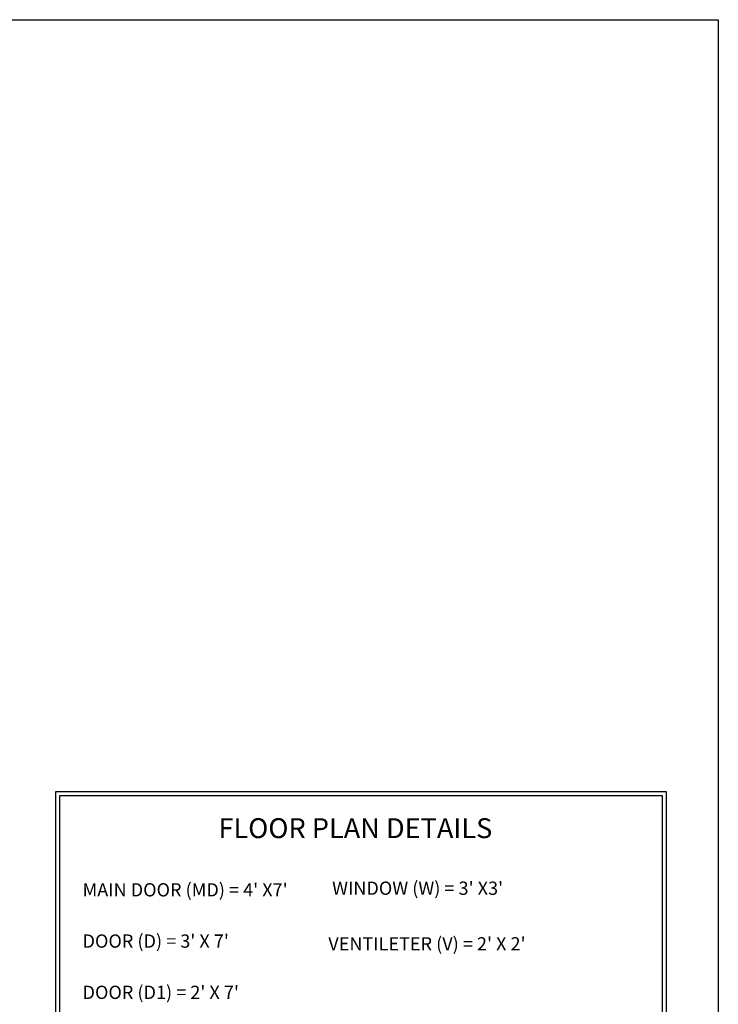
# Model space of a CAD drawing. Units: inches. Extents: x 1662 to 23131, y 1265 to 19127.
# Tile 26 of 26: x 22604 to 23131, y 18361 to 19104. Entities that reach past the tile are written whole.
import ezdxf

# ---------------------------------------------------------------- set-up
doc = ezdxf.new("R2010")
doc.units = ezdxf.units.IN
for name, color, linetype, lineweight in [('A-ANNO-TEXT', 7, 'Continuous', 18), ('A-ANNO-TITL', 7, 'Continuous', 35), ('A-ANNO-TTLB', 7, 'Continuous', 25)]:
    doc.layers.add(name, color=color, linetype=linetype, lineweight=lineweight)
doc.styles.get("Standard").update_dxf_attribs({"font": 'arial.ttf'})

# ---------------------------------------------------------------- blocks, each defined once
blk = doc.blocks.new('SCHEDULE-FRAME')
for points in [[(0, 206.36), (460.01, 206.36), (460.01, 0), (0, 0)], [(3, 203.36), (457.01, 203.36), (457.01, 3), (3, 3)]]:
    blk.add_lwpolyline(points, close=True)

msp = doc.modelspace()

# ---------------------------------------------------------------- linework, layer by layer
at = {"layer": 'A-ANNO-TTLB'}
msp.add_lwpolyline([(21860.989, 19103.605), (23130.86, 19103.605), (23130.86, 17867.351), (21860.989, 17867.351)], close=True, dxfattribs=at)

# ---------------------------------------------------------------- block references
msp.add_blockref('SCHEDULE-FRAME', (22631.532, 18315.105), dxfattribs=at)

# ---------------------------------------------------------------- texts
at = {"layer": 'A-ANNO-TEXT', "char_height": 10, "attachment_point": 1}
for s, insert in [("MAIN DOOR (MD) = 4' X7'", (22651.685, 18452.431)), ("WINDOW (W) = 3' X3'", (22839.8, 18453.651)), ("DOOR (D) = 3' X 7'", (22651.685, 18413.779)), ("VENTILETER (V) = 2' X 2'", (22836.915, 18411.721)), ("DOOR (D1) = 2' X 7'", (22651.685, 18375.127))]:
    msp.add_mtext_dynamic_manual_height_columns(s, width=1142.59551, gutter_width=12.5, heights=[0], dxfattribs=dict(at, insert=insert))
at = {"layer": 'A-ANNO-TITL', "insert": (22754.132, 18501.417), "char_height": 15, "attachment_point": 1}
msp.add_mtext_dynamic_manual_height_columns('FLOOR PLAN DETAILS', width=1142.59551, gutter_width=12.5, heights=[0], dxfattribs=at)

doc.saveas('drawing.dxf')
